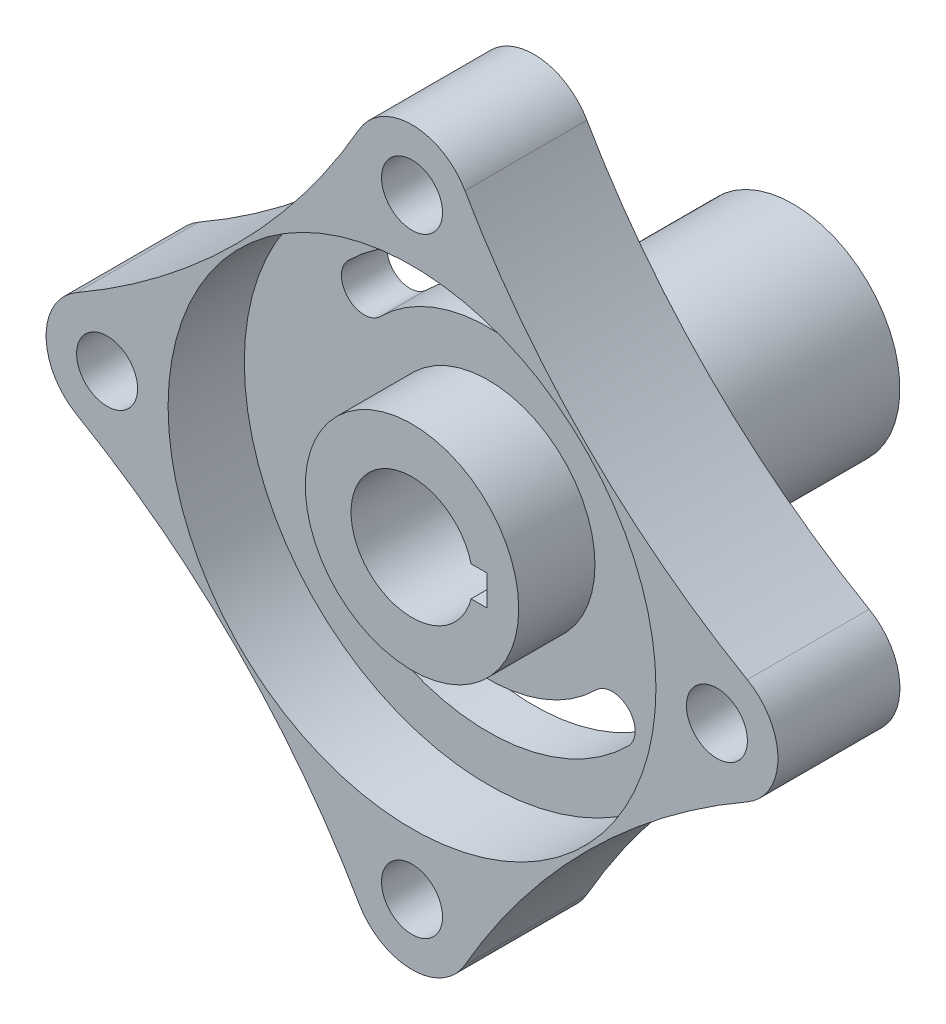
ISO-10303-21;
HEADER;
FILE_DESCRIPTION(('STEP AP214'),'2;1');
FILE_NAME('part.step','',(''),(''),'','','');
FILE_SCHEMA(('AUTOMOTIVE_DESIGN { 1 0 10303 214 1 1 1 1 }'));
ENDSEC;
DATA;
#1=APPLICATION_CONTEXT('core data for automotive mechanical design processes');
#2=APPLICATION_PROTOCOL_DEFINITION('international standard','automotive_design',2000,#1);
#3=PRODUCT_CONTEXT('',#1,'mechanical');
#4=PRODUCT('Part','Part','',(#3));
#5=PRODUCT_RELATED_PRODUCT_CATEGORY('part','',(#4));
#6=PRODUCT_DEFINITION_FORMATION('','',#4);
#7=PRODUCT_DEFINITION_CONTEXT('part definition',#1,'design');
#8=PRODUCT_DEFINITION('design','',#6,#7);
#9=PRODUCT_DEFINITION_SHAPE('','',#8);
#10=(LENGTH_UNIT() NAMED_UNIT(*) SI_UNIT(.MILLI.,.METRE.));
#11=(NAMED_UNIT(*) PLANE_ANGLE_UNIT() SI_UNIT($,.RADIAN.));
#12=(NAMED_UNIT(*) SI_UNIT($,.STERADIAN.) SOLID_ANGLE_UNIT());
#13=UNCERTAINTY_MEASURE_WITH_UNIT(LENGTH_MEASURE(1.E-05),#10,'distance_accuracy_value','');
#14=(GEOMETRIC_REPRESENTATION_CONTEXT(3) GLOBAL_UNCERTAINTY_ASSIGNED_CONTEXT((#13)) GLOBAL_UNIT_ASSIGNED_CONTEXT((#10,
#11,#12)) REPRESENTATION_CONTEXT('',''));
#15=CARTESIAN_POINT('',(0.,0.,0.));
#16=DIRECTION('',(0.,0.,1.));
#17=DIRECTION('',(1.,0.,0.));
#18=AXIS2_PLACEMENT_3D('',#15,#16,#17);
#19=CARTESIAN_POINT('',(0.,0.,0.));
#20=DIRECTION('',(0.,0.,1.));
#21=DIRECTION('',(1.,0.,0.));
#22=AXIS2_PLACEMENT_3D('',#19,#20,#21);
#23=PLANE('',#22);
#24=CARTESIAN_POINT('',(0.,0.,0.));
#25=DIRECTION('',(0.,0.,-1.));
#26=DIRECTION('',(-1.,0.,0.));
#27=AXIS2_PLACEMENT_3D('',#24,#25,#26);
#28=CIRCLE('',#27,14.);
#29=CARTESIAN_POINT('',(-14.,0.,0.));
#30=VERTEX_POINT('',#29);
#31=EDGE_CURVE('E11',#30,#30,#28,.T.);
#32=ORIENTED_EDGE('',*,*,#31,.F.);
#33=EDGE_LOOP('',(#32));
#34=FACE_BOUND('',#33,.T.);
#35=CARTESIAN_POINT('',(-93.7021030907532,-93.7021030907531,0.));
#36=DIRECTION('',(0.,0.,1.));
#37=DIRECTION('',(1.,0.,0.));
#38=AXIS2_PLACEMENT_3D('',#35,#36,#37);
#39=CIRCLE('',#38,100.);
#40=CARTESIAN_POINT('',(-6.94089652524097,-43.977933562278,0.));
#41=VERTEX_POINT('',#40);
#42=CARTESIAN_POINT('',(-43.9779335622782,-6.94089652524068,0.));
#43=VERTEX_POINT('',#42);
#44=EDGE_CURVE('E300',#41,#43,#39,.T.);
#45=ORIENTED_EDGE('',*,*,#44,.T.);
#46=CARTESIAN_POINT('',(-40.,0.,0.));
#47=DIRECTION('',(0.,0.,1.));
#48=DIRECTION('',(1.,0.,0.));
#49=AXIS2_PLACEMENT_3D('',#46,#47,#48);
#50=CIRCLE('',#49,7.99999999999983);
#51=CARTESIAN_POINT('',(-43.9779335622779,6.94089652524083,0.));
#52=VERTEX_POINT('',#51);
#53=EDGE_CURVE('E352',#52,#43,#50,.T.);
#54=ORIENTED_EDGE('',*,*,#53,.F.);
#55=CARTESIAN_POINT('',(-93.7021030907531,93.7021030907531,0.));
#56=DIRECTION('',(0.,0.,1.));
#57=DIRECTION('',(1.,0.,0.));
#58=AXIS2_PLACEMENT_3D('',#55,#56,#57);
#59=CIRCLE('',#58,100.);
#60=CARTESIAN_POINT('',(-6.94089652524097,43.977933562278,0.));
#61=VERTEX_POINT('',#60);
#62=EDGE_CURVE('E353',#52,#61,#59,.T.);
#63=ORIENTED_EDGE('',*,*,#62,.T.);
#64=CARTESIAN_POINT('',(0.,40.,0.));
#65=DIRECTION('',(0.,0.,1.));
#66=DIRECTION('',(1.,0.,0.));
#67=AXIS2_PLACEMENT_3D('',#64,#65,#66);
#68=CIRCLE('',#67,8.);
#69=CARTESIAN_POINT('',(6.94089652524097,43.977933562278,0.));
#70=VERTEX_POINT('',#69);
#71=EDGE_CURVE('E346',#70,#61,#68,.T.);
#72=ORIENTED_EDGE('',*,*,#71,.F.);
#73=CARTESIAN_POINT('',(93.7021030907531,93.7021030907531,0.));
#74=DIRECTION('',(0.,0.,1.));
#75=DIRECTION('',(1.,0.,0.));
#76=AXIS2_PLACEMENT_3D('',#73,#74,#75);
#77=CIRCLE('',#76,100.);
#78=CARTESIAN_POINT('',(43.977933562278,6.94089652524094,0.));
#79=VERTEX_POINT('',#78);
#80=EDGE_CURVE('E344',#70,#79,#77,.T.);
#81=ORIENTED_EDGE('',*,*,#80,.T.);
#82=CARTESIAN_POINT('',(40.,0.,0.));
#83=DIRECTION('',(0.,0.,1.));
#84=DIRECTION('',(1.,0.,0.));
#85=AXIS2_PLACEMENT_3D('',#82,#83,#84);
#86=CIRCLE('',#85,7.99999999999997);
#87=CARTESIAN_POINT('',(43.977933562278,-6.94089652524095,0.));
#88=VERTEX_POINT('',#87);
#89=EDGE_CURVE('E345',#88,#79,#86,.T.);
#90=ORIENTED_EDGE('',*,*,#89,.F.);
#91=CARTESIAN_POINT('',(93.7021030907531,-93.7021030907531,0.));
#92=DIRECTION('',(0.,0.,1.));
#93=DIRECTION('',(1.,0.,0.));
#94=AXIS2_PLACEMENT_3D('',#91,#92,#93);
#95=CIRCLE('',#94,100.);
#96=CARTESIAN_POINT('',(6.94089652524096,-43.977933562278,0.));
#97=VERTEX_POINT('',#96);
#98=EDGE_CURVE('E337',#88,#97,#95,.T.);
#99=ORIENTED_EDGE('',*,*,#98,.T.);
#100=CARTESIAN_POINT('',(0.,-40.,0.));
#101=DIRECTION('',(0.,0.,1.));
#102=DIRECTION('',(1.,0.,0.));
#103=AXIS2_PLACEMENT_3D('',#100,#101,#102);
#104=CIRCLE('',#103,8.);
#105=EDGE_CURVE('E338',#41,#97,#104,.T.);
#106=ORIENTED_EDGE('',*,*,#105,.F.);
#107=EDGE_LOOP('',(#45,#54,#63,#72,#81,#90,#99,#106));
#108=FACE_BOUND('',#107,.T.);
#109=CARTESIAN_POINT('',(0.,-40.,0.));
#110=DIRECTION('',(0.,0.,1.));
#111=DIRECTION('',(1.,0.,0.));
#112=AXIS2_PLACEMENT_3D('',#109,#110,#111);
#113=CIRCLE('',#112,4.);
#114=CARTESIAN_POINT('',(4.,-40.,0.));
#115=VERTEX_POINT('',#114);
#116=EDGE_CURVE('E360',#115,#115,#113,.T.);
#117=ORIENTED_EDGE('',*,*,#116,.T.);
#118=EDGE_LOOP('',(#117));
#119=FACE_BOUND('',#118,.T.);
#120=CARTESIAN_POINT('',(-40.,0.,0.));
#121=DIRECTION('',(0.,0.,1.));
#122=DIRECTION('',(1.,0.,0.));
#123=AXIS2_PLACEMENT_3D('',#120,#121,#122);
#124=CIRCLE('',#123,4.);
#125=CARTESIAN_POINT('',(-36.,0.,0.));
#126=VERTEX_POINT('',#125);
#127=EDGE_CURVE('E359',#126,#126,#124,.T.);
#128=ORIENTED_EDGE('',*,*,#127,.T.);
#129=EDGE_LOOP('',(#128));
#130=FACE_BOUND('',#129,.T.);
#131=CARTESIAN_POINT('',(40.,0.,0.));
#132=DIRECTION('',(0.,0.,1.));
#133=DIRECTION('',(1.,0.,0.));
#134=AXIS2_PLACEMENT_3D('',#131,#132,#133);
#135=CIRCLE('',#134,4.);
#136=CARTESIAN_POINT('',(44.,0.,0.));
#137=VERTEX_POINT('',#136);
#138=EDGE_CURVE('E361',#137,#137,#135,.T.);
#139=ORIENTED_EDGE('',*,*,#138,.T.);
#140=EDGE_LOOP('',(#139));
#141=FACE_BOUND('',#140,.T.);
#142=CARTESIAN_POINT('',(0.,40.,0.));
#143=DIRECTION('',(0.,0.,1.));
#144=DIRECTION('',(1.,0.,0.));
#145=AXIS2_PLACEMENT_3D('',#142,#143,#144);
#146=CIRCLE('',#145,4.);
#147=CARTESIAN_POINT('',(4.,40.,0.));
#148=VERTEX_POINT('',#147);
#149=EDGE_CURVE('E302',#148,#148,#146,.T.);
#150=ORIENTED_EDGE('',*,*,#149,.T.);
#151=EDGE_LOOP('',(#150));
#152=FACE_BOUND('',#151,.T.);
#153=CARTESIAN_POINT('',(0.,0.,0.));
#154=DIRECTION('',(0.,0.,1.));
#155=DIRECTION('',(1.,0.,0.));
#156=AXIS2_PLACEMENT_3D('',#153,#154,#155);
#157=CIRCLE('',#156,26.);
#158=CARTESIAN_POINT('',(18.3847763108502,18.3847763108503,0.));
#159=VERTEX_POINT('',#158);
#160=CARTESIAN_POINT('',(-18.3847763108502,18.3847763108503,0.));
#161=VERTEX_POINT('',#160);
#162=EDGE_CURVE('E273',#159,#161,#157,.T.);
#163=ORIENTED_EDGE('',*,*,#162,.T.);
#164=CARTESIAN_POINT('',(-16.2634559672906,16.2634559672906,0.));
#165=DIRECTION('',(0.,0.,1.));
#166=DIRECTION('',(1.,0.,0.));
#167=AXIS2_PLACEMENT_3D('',#164,#165,#166);
#168=CIRCLE('',#167,3.);
#169=CARTESIAN_POINT('',(-14.1421356237309,14.142135623731,0.));
#170=VERTEX_POINT('',#169);
#171=EDGE_CURVE('E262',#161,#170,#168,.T.);
#172=ORIENTED_EDGE('',*,*,#171,.T.);
#173=CARTESIAN_POINT('',(0.,0.,0.));
#174=DIRECTION('',(0.,0.,-1.));
#175=DIRECTION('',(1.,0.,0.));
#176=AXIS2_PLACEMENT_3D('',#173,#174,#175);
#177=CIRCLE('',#176,20.);
#178=CARTESIAN_POINT('',(14.1421356237309,14.142135623731,0.));
#179=VERTEX_POINT('',#178);
#180=EDGE_CURVE('E270',#170,#179,#177,.T.);
#181=ORIENTED_EDGE('',*,*,#180,.T.);
#182=CARTESIAN_POINT('',(16.2634559672906,16.2634559672906,0.));
#183=DIRECTION('',(0.,0.,1.));
#184=DIRECTION('',(1.,0.,0.));
#185=AXIS2_PLACEMENT_3D('',#182,#183,#184);
#186=CIRCLE('',#185,3.);
#187=EDGE_CURVE('E271',#179,#159,#186,.T.);
#188=ORIENTED_EDGE('',*,*,#187,.T.);
#189=EDGE_LOOP('',(#163,#172,#181,#188));
#190=FACE_BOUND('',#189,.T.);
#191=CARTESIAN_POINT('',(0.,0.,0.));
#192=DIRECTION('',(0.,0.,-1.));
#193=DIRECTION('',(1.,0.,0.));
#194=AXIS2_PLACEMENT_3D('',#191,#192,#193);
#195=CIRCLE('',#194,20.);
#196=CARTESIAN_POINT('',(14.1421356237309,-14.142135623731,0.));
#197=VERTEX_POINT('',#196);
#198=CARTESIAN_POINT('',(-14.1421356237309,-14.142135623731,0.));
#199=VERTEX_POINT('',#198);
#200=EDGE_CURVE('E238',#197,#199,#195,.T.);
#201=ORIENTED_EDGE('',*,*,#200,.T.);
#202=CARTESIAN_POINT('',(-16.2634559672906,-16.2634559672906,0.));
#203=DIRECTION('',(0.,0.,1.));
#204=DIRECTION('',(-1.,0.,0.));
#205=AXIS2_PLACEMENT_3D('',#202,#203,#204);
#206=CIRCLE('',#205,3.);
#207=CARTESIAN_POINT('',(-18.3847763108502,-18.3847763108503,0.));
#208=VERTEX_POINT('',#207);
#209=EDGE_CURVE('E235',#199,#208,#206,.T.);
#210=ORIENTED_EDGE('',*,*,#209,.T.);
#211=CARTESIAN_POINT('',(0.,0.,0.));
#212=DIRECTION('',(0.,0.,1.));
#213=DIRECTION('',(1.,0.,0.));
#214=AXIS2_PLACEMENT_3D('',#211,#212,#213);
#215=CIRCLE('',#214,26.);
#216=CARTESIAN_POINT('',(18.3847763108502,-18.3847763108503,0.));
#217=VERTEX_POINT('',#216);
#218=EDGE_CURVE('E234',#208,#217,#215,.T.);
#219=ORIENTED_EDGE('',*,*,#218,.T.);
#220=CARTESIAN_POINT('',(16.2634559672906,-16.2634559672906,0.));
#221=DIRECTION('',(0.,0.,1.));
#222=DIRECTION('',(1.,0.,0.));
#223=AXIS2_PLACEMENT_3D('',#220,#221,#222);
#224=CIRCLE('',#223,3.);
#225=EDGE_CURVE('E72',#217,#197,#224,.T.);
#226=ORIENTED_EDGE('',*,*,#225,.T.);
#227=EDGE_LOOP('',(#201,#210,#219,#226));
#228=FACE_BOUND('',#227,.T.);
#229=ADVANCED_FACE('F50',(#34,#108,#119,#130,#141,#152,#190,#228),#23,.F.);
#230=CARTESIAN_POINT('',(0.,0.,6.));
#231=DIRECTION('',(0.,0.,1.));
#232=DIRECTION('',(1.,0.,0.));
#233=AXIS2_PLACEMENT_3D('',#230,#231,#232);
#234=PLANE('',#233);
#235=CARTESIAN_POINT('',(0.,0.,6.));
#236=DIRECTION('',(0.,0.,1.));
#237=DIRECTION('',(1.,0.,0.));
#238=AXIS2_PLACEMENT_3D('',#235,#236,#237);
#239=CIRCLE('',#238,14.);
#240=CARTESIAN_POINT('',(14.,0.,6.));
#241=VERTEX_POINT('',#240);
#242=EDGE_CURVE('E221',#241,#241,#239,.T.);
#243=ORIENTED_EDGE('',*,*,#242,.F.);
#244=EDGE_LOOP('',(#243));
#245=FACE_BOUND('',#244,.T.);
#246=CARTESIAN_POINT('',(-16.2634559672906,16.2634559672906,6.));
#247=DIRECTION('',(0.,0.,1.));
#248=DIRECTION('',(1.,0.,0.));
#249=AXIS2_PLACEMENT_3D('',#246,#247,#248);
#250=CIRCLE('',#249,3.);
#251=CARTESIAN_POINT('',(-18.3847763108502,18.3847763108503,6.));
#252=VERTEX_POINT('',#251);
#253=CARTESIAN_POINT('',(-14.1421356237309,14.142135623731,6.));
#254=VERTEX_POINT('',#253);
#255=EDGE_CURVE('E227',#252,#254,#250,.T.);
#256=ORIENTED_EDGE('',*,*,#255,.F.);
#257=CARTESIAN_POINT('',(0.,0.,6.));
#258=DIRECTION('',(0.,0.,1.));
#259=DIRECTION('',(1.,0.,0.));
#260=AXIS2_PLACEMENT_3D('',#257,#258,#259);
#261=CIRCLE('',#260,26.);
#262=CARTESIAN_POINT('',(18.3847763108502,18.3847763108503,6.));
#263=VERTEX_POINT('',#262);
#264=EDGE_CURVE('E268',#263,#252,#261,.T.);
#265=ORIENTED_EDGE('',*,*,#264,.F.);
#266=CARTESIAN_POINT('',(16.2634559672906,16.2634559672906,6.));
#267=DIRECTION('',(0.,0.,1.));
#268=DIRECTION('',(1.,0.,0.));
#269=AXIS2_PLACEMENT_3D('',#266,#267,#268);
#270=CIRCLE('',#269,3.);
#271=CARTESIAN_POINT('',(14.1421356237309,14.142135623731,6.));
#272=VERTEX_POINT('',#271);
#273=EDGE_CURVE('E285',#272,#263,#270,.T.);
#274=ORIENTED_EDGE('',*,*,#273,.F.);
#275=CARTESIAN_POINT('',(0.,0.,6.));
#276=DIRECTION('',(0.,0.,-1.));
#277=DIRECTION('',(1.,0.,0.));
#278=AXIS2_PLACEMENT_3D('',#275,#276,#277);
#279=CIRCLE('',#278,20.);
#280=EDGE_CURVE('E276',#254,#272,#279,.T.);
#281=ORIENTED_EDGE('',*,*,#280,.F.);
#282=EDGE_LOOP('',(#256,#265,#274,#281));
#283=FACE_BOUND('',#282,.T.);
#284=CARTESIAN_POINT('',(0.,0.,6.));
#285=DIRECTION('',(0.,0.,1.));
#286=DIRECTION('',(1.,0.,0.));
#287=AXIS2_PLACEMENT_3D('',#284,#285,#286);
#288=CIRCLE('',#287,32.);
#289=CARTESIAN_POINT('',(32.,0.,6.));
#290=VERTEX_POINT('',#289);
#291=EDGE_CURVE('E294',#290,#290,#288,.T.);
#292=ORIENTED_EDGE('',*,*,#291,.T.);
#293=EDGE_LOOP('',(#292));
#294=FACE_BOUND('',#293,.T.);
#295=CARTESIAN_POINT('',(-16.2634559672906,-16.2634559672906,6.));
#296=DIRECTION('',(0.,0.,1.));
#297=DIRECTION('',(-1.,0.,0.));
#298=AXIS2_PLACEMENT_3D('',#295,#296,#297);
#299=CIRCLE('',#298,3.);
#300=CARTESIAN_POINT('',(-14.1421356237309,-14.142135623731,6.));
#301=VERTEX_POINT('',#300);
#302=CARTESIAN_POINT('',(-18.3847763108502,-18.3847763108503,6.));
#303=VERTEX_POINT('',#302);
#304=EDGE_CURVE('E242',#301,#303,#299,.T.);
#305=ORIENTED_EDGE('',*,*,#304,.F.);
#306=CARTESIAN_POINT('',(0.,0.,6.));
#307=DIRECTION('',(0.,0.,-1.));
#308=DIRECTION('',(1.,0.,0.));
#309=AXIS2_PLACEMENT_3D('',#306,#307,#308);
#310=CIRCLE('',#309,20.);
#311=CARTESIAN_POINT('',(14.1421356237309,-14.142135623731,6.));
#312=VERTEX_POINT('',#311);
#313=EDGE_CURVE('E237',#312,#301,#310,.T.);
#314=ORIENTED_EDGE('',*,*,#313,.F.);
#315=CARTESIAN_POINT('',(16.2634559672906,-16.2634559672906,6.));
#316=DIRECTION('',(0.,0.,1.));
#317=DIRECTION('',(1.,0.,0.));
#318=AXIS2_PLACEMENT_3D('',#315,#316,#317);
#319=CIRCLE('',#318,3.);
#320=CARTESIAN_POINT('',(18.3847763108502,-18.3847763108503,6.));
#321=VERTEX_POINT('',#320);
#322=EDGE_CURVE('E249',#321,#312,#319,.T.);
#323=ORIENTED_EDGE('',*,*,#322,.F.);
#324=CARTESIAN_POINT('',(0.,0.,6.));
#325=DIRECTION('',(0.,0.,1.));
#326=DIRECTION('',(1.,0.,0.));
#327=AXIS2_PLACEMENT_3D('',#324,#325,#326);
#328=CIRCLE('',#327,26.);
#329=EDGE_CURVE('E246',#303,#321,#328,.T.);
#330=ORIENTED_EDGE('',*,*,#329,.F.);
#331=EDGE_LOOP('',(#305,#314,#323,#330));
#332=FACE_BOUND('',#331,.T.);
#333=ADVANCED_FACE('F438',(#245,#283,#294,#332),#234,.T.);
#334=CARTESIAN_POINT('',(-93.7021030907532,-93.7021030907531,16.));
#335=DIRECTION('',(0.,0.,-1.));
#336=DIRECTION('',(-1.,0.,0.));
#337=AXIS2_PLACEMENT_3D('',#334,#335,#336);
#338=CYLINDRICAL_SURFACE('',#337,100.);
#339=ORIENTED_EDGE('',*,*,#44,.F.);
#340=DIRECTION('',(0.,0.,-1.));
#341=VECTOR('',#340,1.);
#342=CARTESIAN_POINT('',(-6.94089652524097,-43.977933562278,16.));
#343=LINE('',#342,#341);
#344=CARTESIAN_POINT('',(-6.94089652524097,-43.977933562278,16.));
#345=VERTEX_POINT('',#344);
#346=EDGE_CURVE('E51',#345,#41,#343,.T.);
#347=ORIENTED_EDGE('',*,*,#346,.F.);
#348=CARTESIAN_POINT('',(-93.7021030907532,-93.7021030907531,16.));
#349=DIRECTION('',(0.,0.,1.));
#350=DIRECTION('',(1.,0.,0.));
#351=AXIS2_PLACEMENT_3D('',#348,#349,#350);
#352=CIRCLE('',#351,100.);
#353=CARTESIAN_POINT('',(-43.9779335622782,-6.94089652524068,16.));
#354=VERTEX_POINT('',#353);
#355=EDGE_CURVE('E299',#345,#354,#352,.T.);
#356=ORIENTED_EDGE('',*,*,#355,.T.);
#357=DIRECTION('',(0.,0.,-1.));
#358=VECTOR('',#357,1.);
#359=CARTESIAN_POINT('',(-43.9779335622782,-6.94089652524068,16.));
#360=LINE('',#359,#358);
#361=EDGE_CURVE('E334',#354,#43,#360,.T.);
#362=ORIENTED_EDGE('',*,*,#361,.T.);
#363=EDGE_LOOP('',(#339,#347,#356,#362));
#364=FACE_BOUND('',#363,.T.);
#365=ADVANCED_FACE('F47',(#364),#338,.F.);
#366=CARTESIAN_POINT('',(0.,-40.,16.));
#367=DIRECTION('',(0.,0.,-1.));
#368=DIRECTION('',(-1.,0.,0.));
#369=AXIS2_PLACEMENT_3D('',#366,#367,#368);
#370=CYLINDRICAL_SURFACE('',#369,8.);
#371=ORIENTED_EDGE('',*,*,#105,.T.);
#372=DIRECTION('',(0.,0.,-1.));
#373=VECTOR('',#372,1.);
#374=CARTESIAN_POINT('',(6.94089652524096,-43.977933562278,16.));
#375=LINE('',#374,#373);
#376=CARTESIAN_POINT('',(6.94089652524096,-43.977933562278,16.));
#377=VERTEX_POINT('',#376);
#378=EDGE_CURVE('E378',#377,#97,#375,.T.);
#379=ORIENTED_EDGE('',*,*,#378,.F.);
#380=CARTESIAN_POINT('',(0.,-40.,16.));
#381=DIRECTION('',(0.,0.,1.));
#382=DIRECTION('',(1.,0.,0.));
#383=AXIS2_PLACEMENT_3D('',#380,#381,#382);
#384=CIRCLE('',#383,8.);
#385=EDGE_CURVE('E303',#345,#377,#384,.T.);
#386=ORIENTED_EDGE('',*,*,#385,.F.);
#387=ORIENTED_EDGE('',*,*,#346,.T.);
#388=EDGE_LOOP('',(#371,#379,#386,#387));
#389=FACE_BOUND('',#388,.T.);
#390=ADVANCED_FACE('F384',(#389),#370,.T.);
#391=CARTESIAN_POINT('',(93.7021030907531,-93.7021030907531,16.));
#392=DIRECTION('',(0.,0.,-1.));
#393=DIRECTION('',(-1.,0.,0.));
#394=AXIS2_PLACEMENT_3D('',#391,#392,#393);
#395=CYLINDRICAL_SURFACE('',#394,100.);
#396=ORIENTED_EDGE('',*,*,#98,.F.);
#397=DIRECTION('',(0.,0.,-1.));
#398=VECTOR('',#397,1.);
#399=CARTESIAN_POINT('',(43.977933562278,-6.94089652524095,16.));
#400=LINE('',#399,#398);
#401=CARTESIAN_POINT('',(43.977933562278,-6.94089652524095,16.));
#402=VERTEX_POINT('',#401);
#403=EDGE_CURVE('E380',#402,#88,#400,.T.);
#404=ORIENTED_EDGE('',*,*,#403,.F.);
#405=CARTESIAN_POINT('',(93.7021030907531,-93.7021030907531,16.));
#406=DIRECTION('',(0.,0.,1.));
#407=DIRECTION('',(1.,0.,0.));
#408=AXIS2_PLACEMENT_3D('',#405,#406,#407);
#409=CIRCLE('',#408,100.);
#410=EDGE_CURVE('E308',#402,#377,#409,.T.);
#411=ORIENTED_EDGE('',*,*,#410,.T.);
#412=ORIENTED_EDGE('',*,*,#378,.T.);
#413=EDGE_LOOP('',(#396,#404,#411,#412));
#414=FACE_BOUND('',#413,.T.);
#415=ADVANCED_FACE('F412',(#414),#395,.F.);
#416=CARTESIAN_POINT('',(40.,0.,16.));
#417=DIRECTION('',(0.,0.,-1.));
#418=DIRECTION('',(-1.,0.,0.));
#419=AXIS2_PLACEMENT_3D('',#416,#417,#418);
#420=CYLINDRICAL_SURFACE('',#419,7.99999999999997);
#421=ORIENTED_EDGE('',*,*,#89,.T.);
#422=DIRECTION('',(0.,0.,-1.));
#423=VECTOR('',#422,1.);
#424=CARTESIAN_POINT('',(43.977933562278,6.94089652524094,16.));
#425=LINE('',#424,#423);
#426=CARTESIAN_POINT('',(43.977933562278,6.94089652524094,16.));
#427=VERTEX_POINT('',#426);
#428=EDGE_CURVE('E374',#427,#79,#425,.T.);
#429=ORIENTED_EDGE('',*,*,#428,.F.);
#430=CARTESIAN_POINT('',(40.,0.,16.));
#431=DIRECTION('',(0.,0.,1.));
#432=DIRECTION('',(1.,0.,0.));
#433=AXIS2_PLACEMENT_3D('',#430,#431,#432);
#434=CIRCLE('',#433,7.99999999999997);
#435=EDGE_CURVE('E310',#402,#427,#434,.T.);
#436=ORIENTED_EDGE('',*,*,#435,.F.);
#437=ORIENTED_EDGE('',*,*,#403,.T.);
#438=EDGE_LOOP('',(#421,#429,#436,#437));
#439=FACE_BOUND('',#438,.T.);
#440=ADVANCED_FACE('F413',(#439),#420,.T.);
#441=CARTESIAN_POINT('',(93.7021030907531,93.7021030907531,16.));
#442=DIRECTION('',(0.,0.,-1.));
#443=DIRECTION('',(-1.,0.,0.));
#444=AXIS2_PLACEMENT_3D('',#441,#442,#443);
#445=CYLINDRICAL_SURFACE('',#444,100.);
#446=ORIENTED_EDGE('',*,*,#80,.F.);
#447=DIRECTION('',(0.,0.,-1.));
#448=VECTOR('',#447,1.);
#449=CARTESIAN_POINT('',(6.94089652524097,43.977933562278,16.));
#450=LINE('',#449,#448);
#451=CARTESIAN_POINT('',(6.94089652524097,43.977933562278,16.));
#452=VERTEX_POINT('',#451);
#453=EDGE_CURVE('E373',#452,#70,#450,.T.);
#454=ORIENTED_EDGE('',*,*,#453,.F.);
#455=CARTESIAN_POINT('',(93.7021030907531,93.7021030907531,16.));
#456=DIRECTION('',(0.,0.,1.));
#457=DIRECTION('',(1.,0.,0.));
#458=AXIS2_PLACEMENT_3D('',#455,#456,#457);
#459=CIRCLE('',#458,100.);
#460=EDGE_CURVE('E313',#452,#427,#459,.T.);
#461=ORIENTED_EDGE('',*,*,#460,.T.);
#462=ORIENTED_EDGE('',*,*,#428,.T.);
#463=EDGE_LOOP('',(#446,#454,#461,#462));
#464=FACE_BOUND('',#463,.T.);
#465=ADVANCED_FACE('F406',(#464),#445,.F.);
#466=CARTESIAN_POINT('',(0.,40.,16.));
#467=DIRECTION('',(0.,0.,-1.));
#468=DIRECTION('',(-1.,0.,0.));
#469=AXIS2_PLACEMENT_3D('',#466,#467,#468);
#470=CYLINDRICAL_SURFACE('',#469,8.);
#471=ORIENTED_EDGE('',*,*,#71,.T.);
#472=DIRECTION('',(0.,0.,-1.));
#473=VECTOR('',#472,1.);
#474=CARTESIAN_POINT('',(-6.94089652524097,43.977933562278,16.));
#475=LINE('',#474,#473);
#476=CARTESIAN_POINT('',(-6.94089652524097,43.977933562278,16.));
#477=VERTEX_POINT('',#476);
#478=EDGE_CURVE('E371',#477,#61,#475,.T.);
#479=ORIENTED_EDGE('',*,*,#478,.F.);
#480=CARTESIAN_POINT('',(0.,40.,16.));
#481=DIRECTION('',(0.,0.,1.));
#482=DIRECTION('',(1.,0.,0.));
#483=AXIS2_PLACEMENT_3D('',#480,#481,#482);
#484=CIRCLE('',#483,8.);
#485=EDGE_CURVE('E314',#452,#477,#484,.T.);
#486=ORIENTED_EDGE('',*,*,#485,.F.);
#487=ORIENTED_EDGE('',*,*,#453,.T.);
#488=EDGE_LOOP('',(#471,#479,#486,#487));
#489=FACE_BOUND('',#488,.T.);
#490=ADVANCED_FACE('F403',(#489),#470,.T.);
#491=CARTESIAN_POINT('',(-93.7021030907531,93.7021030907531,16.));
#492=DIRECTION('',(0.,0.,-1.));
#493=DIRECTION('',(-1.,0.,0.));
#494=AXIS2_PLACEMENT_3D('',#491,#492,#493);
#495=CYLINDRICAL_SURFACE('',#494,100.);
#496=ORIENTED_EDGE('',*,*,#62,.F.);
#497=DIRECTION('',(0.,0.,-1.));
#498=VECTOR('',#497,1.);
#499=CARTESIAN_POINT('',(-43.9779335622779,6.94089652524083,16.));
#500=LINE('',#499,#498);
#501=CARTESIAN_POINT('',(-43.9779335622779,6.94089652524083,16.));
#502=VERTEX_POINT('',#501);
#503=EDGE_CURVE('E369',#502,#52,#500,.T.);
#504=ORIENTED_EDGE('',*,*,#503,.F.);
#505=CARTESIAN_POINT('',(-93.7021030907531,93.7021030907531,16.));
#506=DIRECTION('',(0.,0.,1.));
#507=DIRECTION('',(1.,0.,0.));
#508=AXIS2_PLACEMENT_3D('',#505,#506,#507);
#509=CIRCLE('',#508,100.);
#510=EDGE_CURVE('E316',#502,#477,#509,.T.);
#511=ORIENTED_EDGE('',*,*,#510,.T.);
#512=ORIENTED_EDGE('',*,*,#478,.T.);
#513=EDGE_LOOP('',(#496,#504,#511,#512));
#514=FACE_BOUND('',#513,.T.);
#515=ADVANCED_FACE('F399',(#514),#495,.F.);
#516=CARTESIAN_POINT('',(40.,0.,16.));
#517=DIRECTION('',(0.,0.,-1.));
#518=DIRECTION('',(-1.,0.,0.));
#519=AXIS2_PLACEMENT_3D('',#516,#517,#518);
#520=CYLINDRICAL_SURFACE('',#519,4.);
#521=CARTESIAN_POINT('',(40.,0.,16.));
#522=DIRECTION('',(0.,0.,1.));
#523=DIRECTION('',(1.,0.,0.));
#524=AXIS2_PLACEMENT_3D('',#521,#522,#523);
#525=CIRCLE('',#524,4.);
#526=CARTESIAN_POINT('',(44.,0.,16.));
#527=VERTEX_POINT('',#526);
#528=EDGE_CURVE('E330',#527,#527,#525,.T.);
#529=ORIENTED_EDGE('',*,*,#528,.T.);
#530=EDGE_LOOP('',(#529));
#531=FACE_BOUND('',#530,.T.);
#532=ORIENTED_EDGE('',*,*,#138,.F.);
#533=EDGE_LOOP('',(#532));
#534=FACE_BOUND('',#533,.T.);
#535=ADVANCED_FACE('F478',(#531,#534),#520,.F.);
#536=CARTESIAN_POINT('',(-40.,0.,16.));
#537=DIRECTION('',(0.,0.,-1.));
#538=DIRECTION('',(-1.,0.,0.));
#539=AXIS2_PLACEMENT_3D('',#536,#537,#538);
#540=CYLINDRICAL_SURFACE('',#539,4.);
#541=CARTESIAN_POINT('',(-40.,0.,16.));
#542=DIRECTION('',(0.,0.,1.));
#543=DIRECTION('',(1.,0.,0.));
#544=AXIS2_PLACEMENT_3D('',#541,#542,#543);
#545=CIRCLE('',#544,4.);
#546=CARTESIAN_POINT('',(-36.,0.,16.));
#547=VERTEX_POINT('',#546);
#548=EDGE_CURVE('E322',#547,#547,#545,.T.);
#549=ORIENTED_EDGE('',*,*,#548,.T.);
#550=EDGE_LOOP('',(#549));
#551=FACE_BOUND('',#550,.T.);
#552=ORIENTED_EDGE('',*,*,#127,.F.);
#553=EDGE_LOOP('',(#552));
#554=FACE_BOUND('',#553,.T.);
#555=ADVANCED_FACE('F479',(#551,#554),#540,.F.);
#556=CARTESIAN_POINT('',(0.,-40.,16.));
#557=DIRECTION('',(0.,0.,-1.));
#558=DIRECTION('',(-1.,0.,0.));
#559=AXIS2_PLACEMENT_3D('',#556,#557,#558);
#560=CYLINDRICAL_SURFACE('',#559,4.);
#561=CARTESIAN_POINT('',(0.,-40.,16.));
#562=DIRECTION('',(0.,0.,1.));
#563=DIRECTION('',(1.,0.,0.));
#564=AXIS2_PLACEMENT_3D('',#561,#562,#563);
#565=CIRCLE('',#564,4.);
#566=CARTESIAN_POINT('',(4.,-40.,16.));
#567=VERTEX_POINT('',#566);
#568=EDGE_CURVE('E321',#567,#567,#565,.T.);
#569=ORIENTED_EDGE('',*,*,#568,.T.);
#570=EDGE_LOOP('',(#569));
#571=FACE_BOUND('',#570,.T.);
#572=ORIENTED_EDGE('',*,*,#116,.F.);
#573=EDGE_LOOP('',(#572));
#574=FACE_BOUND('',#573,.T.);
#575=ADVANCED_FACE('F483',(#571,#574),#560,.F.);
#576=CARTESIAN_POINT('',(-40.,0.,16.));
#577=DIRECTION('',(0.,0.,-1.));
#578=DIRECTION('',(-1.,0.,0.));
#579=AXIS2_PLACEMENT_3D('',#576,#577,#578);
#580=CYLINDRICAL_SURFACE('',#579,7.99999999999983);
#581=ORIENTED_EDGE('',*,*,#53,.T.);
#582=ORIENTED_EDGE('',*,*,#361,.F.);
#583=CARTESIAN_POINT('',(-40.,0.,16.));
#584=DIRECTION('',(0.,0.,1.));
#585=DIRECTION('',(1.,0.,0.));
#586=AXIS2_PLACEMENT_3D('',#583,#584,#585);
#587=CIRCLE('',#586,7.99999999999983);
#588=EDGE_CURVE('E317',#502,#354,#587,.T.);
#589=ORIENTED_EDGE('',*,*,#588,.F.);
#590=ORIENTED_EDGE('',*,*,#503,.T.);
#591=EDGE_LOOP('',(#581,#582,#589,#590));
#592=FACE_BOUND('',#591,.T.);
#593=ADVANCED_FACE('F396',(#592),#580,.T.);
#594=CARTESIAN_POINT('',(0.,40.,16.));
#595=DIRECTION('',(0.,0.,-1.));
#596=DIRECTION('',(-1.,0.,0.));
#597=AXIS2_PLACEMENT_3D('',#594,#595,#596);
#598=CYLINDRICAL_SURFACE('',#597,4.);
#599=CARTESIAN_POINT('',(0.,40.,16.));
#600=DIRECTION('',(0.,0.,1.));
#601=DIRECTION('',(1.,0.,0.));
#602=AXIS2_PLACEMENT_3D('',#599,#600,#601);
#603=CIRCLE('',#602,4.);
#604=CARTESIAN_POINT('',(4.,40.,16.));
#605=VERTEX_POINT('',#604);
#606=EDGE_CURVE('E329',#605,#605,#603,.T.);
#607=ORIENTED_EDGE('',*,*,#606,.T.);
#608=EDGE_LOOP('',(#607));
#609=FACE_BOUND('',#608,.T.);
#610=ORIENTED_EDGE('',*,*,#149,.F.);
#611=EDGE_LOOP('',(#610));
#612=FACE_BOUND('',#611,.T.);
#613=ADVANCED_FACE('F423',(#609,#612),#598,.F.);
#614=CARTESIAN_POINT('',(0.,0.,16.));
#615=DIRECTION('',(0.,0.,1.));
#616=DIRECTION('',(1.,0.,0.));
#617=AXIS2_PLACEMENT_3D('',#614,#615,#616);
#618=PLANE('',#617);
#619=CARTESIAN_POINT('',(0.,0.,16.));
#620=DIRECTION('',(0.,0.,1.));
#621=DIRECTION('',(1.,0.,0.));
#622=AXIS2_PLACEMENT_3D('',#619,#620,#621);
#623=CIRCLE('',#622,32.);
#624=CARTESIAN_POINT('',(32.,0.,16.));
#625=VERTEX_POINT('',#624);
#626=EDGE_CURVE('E260',#625,#625,#623,.T.);
#627=ORIENTED_EDGE('',*,*,#626,.F.);
#628=EDGE_LOOP('',(#627));
#629=FACE_BOUND('',#628,.T.);
#630=ORIENTED_EDGE('',*,*,#355,.F.);
#631=ORIENTED_EDGE('',*,*,#385,.T.);
#632=ORIENTED_EDGE('',*,*,#410,.F.);
#633=ORIENTED_EDGE('',*,*,#435,.T.);
#634=ORIENTED_EDGE('',*,*,#460,.F.);
#635=ORIENTED_EDGE('',*,*,#485,.T.);
#636=ORIENTED_EDGE('',*,*,#510,.F.);
#637=ORIENTED_EDGE('',*,*,#588,.T.);
#638=EDGE_LOOP('',(#630,#631,#632,#633,#634,#635,#636,#637));
#639=FACE_BOUND('',#638,.T.);
#640=ORIENTED_EDGE('',*,*,#568,.F.);
#641=EDGE_LOOP('',(#640));
#642=FACE_BOUND('',#641,.T.);
#643=ORIENTED_EDGE('',*,*,#548,.F.);
#644=EDGE_LOOP('',(#643));
#645=FACE_BOUND('',#644,.T.);
#646=ORIENTED_EDGE('',*,*,#528,.F.);
#647=EDGE_LOOP('',(#646));
#648=FACE_BOUND('',#647,.T.);
#649=ORIENTED_EDGE('',*,*,#606,.F.);
#650=EDGE_LOOP('',(#649));
#651=FACE_BOUND('',#650,.T.);
#652=ADVANCED_FACE('F417',(#629,#639,#642,#645,#648,#651),#618,.T.);
#653=CARTESIAN_POINT('',(0.,0.,6.));
#654=DIRECTION('',(0.,0.,1.));
#655=DIRECTION('',(1.,0.,0.));
#656=AXIS2_PLACEMENT_3D('',#653,#654,#655);
#657=CYLINDRICAL_SURFACE('',#656,32.);
#658=ORIENTED_EDGE('',*,*,#291,.F.);
#659=EDGE_LOOP('',(#658));
#660=FACE_BOUND('',#659,.T.);
#661=ORIENTED_EDGE('',*,*,#626,.T.);
#662=EDGE_LOOP('',(#661));
#663=FACE_BOUND('',#662,.T.);
#664=ADVANCED_FACE('F419',(#660,#663),#657,.F.);
#665=CARTESIAN_POINT('',(-16.2634559672906,16.2634559672906,0.));
#666=DIRECTION('',(0.,0.,1.));
#667=DIRECTION('',(1.,0.,0.));
#668=AXIS2_PLACEMENT_3D('',#665,#666,#667);
#669=CYLINDRICAL_SURFACE('',#668,3.);
#670=ORIENTED_EDGE('',*,*,#255,.T.);
#671=DIRECTION('',(0.,0.,1.));
#672=VECTOR('',#671,1.);
#673=CARTESIAN_POINT('',(-14.1421356237309,14.142135623731,0.));
#674=LINE('',#673,#672);
#675=EDGE_CURVE('E280',#170,#254,#674,.T.);
#676=ORIENTED_EDGE('',*,*,#675,.F.);
#677=ORIENTED_EDGE('',*,*,#171,.F.);
#678=DIRECTION('',(0.,0.,1.));
#679=VECTOR('',#678,1.);
#680=CARTESIAN_POINT('',(-18.3847763108502,18.3847763108503,0.));
#681=LINE('',#680,#679);
#682=EDGE_CURVE('E250',#161,#252,#681,.T.);
#683=ORIENTED_EDGE('',*,*,#682,.T.);
#684=EDGE_LOOP('',(#670,#676,#677,#683));
#685=FACE_BOUND('',#684,.T.);
#686=ADVANCED_FACE('F473',(#685),#669,.F.);
#687=CARTESIAN_POINT('',(0.,0.,0.));
#688=DIRECTION('',(0.,0.,1.));
#689=DIRECTION('',(1.,0.,0.));
#690=AXIS2_PLACEMENT_3D('',#687,#688,#689);
#691=CYLINDRICAL_SURFACE('',#690,26.);
#692=ORIENTED_EDGE('',*,*,#264,.T.);
#693=ORIENTED_EDGE('',*,*,#682,.F.);
#694=ORIENTED_EDGE('',*,*,#162,.F.);
#695=DIRECTION('',(0.,0.,1.));
#696=VECTOR('',#695,1.);
#697=CARTESIAN_POINT('',(18.3847763108502,18.3847763108503,0.));
#698=LINE('',#697,#696);
#699=EDGE_CURVE('E288',#159,#263,#698,.T.);
#700=ORIENTED_EDGE('',*,*,#699,.T.);
#701=EDGE_LOOP('',(#692,#693,#694,#700));
#702=FACE_BOUND('',#701,.T.);
#703=ADVANCED_FACE('F587',(#702),#691,.F.);
#704=CARTESIAN_POINT('',(16.2634559672906,16.2634559672906,0.));
#705=DIRECTION('',(0.,0.,1.));
#706=DIRECTION('',(1.,0.,0.));
#707=AXIS2_PLACEMENT_3D('',#704,#705,#706);
#708=CYLINDRICAL_SURFACE('',#707,3.);
#709=ORIENTED_EDGE('',*,*,#273,.T.);
#710=ORIENTED_EDGE('',*,*,#699,.F.);
#711=ORIENTED_EDGE('',*,*,#187,.F.);
#712=DIRECTION('',(0.,0.,1.));
#713=VECTOR('',#712,1.);
#714=CARTESIAN_POINT('',(14.1421356237309,14.142135623731,0.));
#715=LINE('',#714,#713);
#716=EDGE_CURVE('E289',#179,#272,#715,.T.);
#717=ORIENTED_EDGE('',*,*,#716,.T.);
#718=EDGE_LOOP('',(#709,#710,#711,#717));
#719=FACE_BOUND('',#718,.T.);
#720=ADVANCED_FACE('F605',(#719),#708,.F.);
#721=CARTESIAN_POINT('',(0.,0.,0.));
#722=DIRECTION('',(0.,0.,1.));
#723=DIRECTION('',(1.,0.,0.));
#724=AXIS2_PLACEMENT_3D('',#721,#722,#723);
#725=CYLINDRICAL_SURFACE('',#724,20.);
#726=ORIENTED_EDGE('',*,*,#280,.T.);
#727=ORIENTED_EDGE('',*,*,#716,.F.);
#728=ORIENTED_EDGE('',*,*,#180,.F.);
#729=ORIENTED_EDGE('',*,*,#675,.T.);
#730=EDGE_LOOP('',(#726,#727,#728,#729));
#731=FACE_BOUND('',#730,.T.);
#732=ADVANCED_FACE('F612',(#731),#725,.T.);
#733=CARTESIAN_POINT('',(-16.2634559672906,-16.2634559672906,0.));
#734=DIRECTION('',(0.,0.,1.));
#735=DIRECTION('',(1.,0.,0.));
#736=AXIS2_PLACEMENT_3D('',#733,#734,#735);
#737=CYLINDRICAL_SURFACE('',#736,3.);
#738=ORIENTED_EDGE('',*,*,#304,.T.);
#739=DIRECTION('',(0.,0.,1.));
#740=VECTOR('',#739,1.);
#741=CARTESIAN_POINT('',(-18.3847763108502,-18.3847763108503,0.));
#742=LINE('',#741,#740);
#743=EDGE_CURVE('E241',#208,#303,#742,.T.);
#744=ORIENTED_EDGE('',*,*,#743,.F.);
#745=ORIENTED_EDGE('',*,*,#209,.F.);
#746=DIRECTION('',(0.,0.,1.));
#747=VECTOR('',#746,1.);
#748=CARTESIAN_POINT('',(-14.1421356237309,-14.142135623731,0.));
#749=LINE('',#748,#747);
#750=EDGE_CURVE('E254',#199,#301,#749,.T.);
#751=ORIENTED_EDGE('',*,*,#750,.T.);
#752=EDGE_LOOP('',(#738,#744,#745,#751));
#753=FACE_BOUND('',#752,.T.);
#754=ADVANCED_FACE('F451',(#753),#737,.F.);
#755=CARTESIAN_POINT('',(0.,0.,0.));
#756=DIRECTION('',(0.,0.,1.));
#757=DIRECTION('',(1.,0.,0.));
#758=AXIS2_PLACEMENT_3D('',#755,#756,#757);
#759=CYLINDRICAL_SURFACE('',#758,20.);
#760=ORIENTED_EDGE('',*,*,#313,.T.);
#761=ORIENTED_EDGE('',*,*,#750,.F.);
#762=ORIENTED_EDGE('',*,*,#200,.F.);
#763=DIRECTION('',(0.,0.,1.));
#764=VECTOR('',#763,1.);
#765=CARTESIAN_POINT('',(14.1421356237309,-14.142135623731,0.));
#766=LINE('',#765,#764);
#767=EDGE_CURVE('E256',#197,#312,#766,.T.);
#768=ORIENTED_EDGE('',*,*,#767,.T.);
#769=EDGE_LOOP('',(#760,#761,#762,#768));
#770=FACE_BOUND('',#769,.T.);
#771=ADVANCED_FACE('F450',(#770),#759,.T.);
#772=CARTESIAN_POINT('',(16.2634559672906,-16.2634559672906,0.));
#773=DIRECTION('',(0.,0.,1.));
#774=DIRECTION('',(1.,0.,0.));
#775=AXIS2_PLACEMENT_3D('',#772,#773,#774);
#776=CYLINDRICAL_SURFACE('',#775,3.);
#777=ORIENTED_EDGE('',*,*,#322,.T.);
#778=ORIENTED_EDGE('',*,*,#767,.F.);
#779=ORIENTED_EDGE('',*,*,#225,.F.);
#780=DIRECTION('',(0.,0.,1.));
#781=VECTOR('',#780,1.);
#782=CARTESIAN_POINT('',(18.3847763108502,-18.3847763108503,0.));
#783=LINE('',#782,#781);
#784=EDGE_CURVE('E257',#217,#321,#783,.T.);
#785=ORIENTED_EDGE('',*,*,#784,.T.);
#786=EDGE_LOOP('',(#777,#778,#779,#785));
#787=FACE_BOUND('',#786,.T.);
#788=ADVANCED_FACE('F460',(#787),#776,.F.);
#789=CARTESIAN_POINT('',(0.,0.,0.));
#790=DIRECTION('',(0.,0.,1.));
#791=DIRECTION('',(1.,0.,0.));
#792=AXIS2_PLACEMENT_3D('',#789,#790,#791);
#793=CYLINDRICAL_SURFACE('',#792,26.);
#794=ORIENTED_EDGE('',*,*,#329,.T.);
#795=ORIENTED_EDGE('',*,*,#784,.F.);
#796=ORIENTED_EDGE('',*,*,#218,.F.);
#797=ORIENTED_EDGE('',*,*,#743,.T.);
#798=EDGE_LOOP('',(#794,#795,#796,#797));
#799=FACE_BOUND('',#798,.T.);
#800=ADVANCED_FACE('F454',(#799),#793,.F.);
#801=CARTESIAN_POINT('',(0.,0.,16.));
#802=DIRECTION('',(0.,0.,-1.));
#803=DIRECTION('',(-1.,0.,0.));
#804=AXIS2_PLACEMENT_3D('',#801,#802,#803);
#805=CYLINDRICAL_SURFACE('',#804,14.);
#806=CARTESIAN_POINT('',(0.,0.,16.));
#807=DIRECTION('',(0.,0.,1.));
#808=DIRECTION('',(1.,0.,0.));
#809=AXIS2_PLACEMENT_3D('',#806,#807,#808);
#810=CIRCLE('',#809,14.);
#811=CARTESIAN_POINT('',(14.,0.,16.));
#812=VERTEX_POINT('',#811);
#813=EDGE_CURVE('E228',#812,#812,#810,.T.);
#814=ORIENTED_EDGE('',*,*,#813,.F.);
#815=EDGE_LOOP('',(#814));
#816=FACE_BOUND('',#815,.T.);
#817=ORIENTED_EDGE('',*,*,#242,.T.);
#818=EDGE_LOOP('',(#817));
#819=FACE_BOUND('',#818,.T.);
#820=ADVANCED_FACE('F661',(#816,#819),#805,.T.);
#821=CARTESIAN_POINT('',(0.,0.,16.));
#822=DIRECTION('',(0.,0.,1.));
#823=DIRECTION('',(1.,0.,0.));
#824=AXIS2_PLACEMENT_3D('',#821,#822,#823);
#825=PLANE('',#824);
#826=CARTESIAN_POINT('',(0.,0.,16.));
#827=DIRECTION('',(0.,0.,1.));
#828=DIRECTION('',(1.,0.,0.));
#829=AXIS2_PLACEMENT_3D('',#826,#827,#828);
#830=CIRCLE('',#829,8.);
#831=CARTESIAN_POINT('',(7.74854179829986,1.99,16.));
#832=VERTEX_POINT('',#831);
#833=CARTESIAN_POINT('',(7.74854179829986,-1.99,16.));
#834=VERTEX_POINT('',#833);
#835=EDGE_CURVE('E61',#832,#834,#830,.T.);
#836=ORIENTED_EDGE('',*,*,#835,.F.);
#837=DIRECTION('',(-1.,0.,0.));
#838=VECTOR('',#837,1.);
#839=CARTESIAN_POINT('',(9.85,1.99,16.));
#840=LINE('',#839,#838);
#841=CARTESIAN_POINT('',(9.85,1.99,16.));
#842=VERTEX_POINT('',#841);
#843=EDGE_CURVE('E204',#842,#832,#840,.T.);
#844=ORIENTED_EDGE('',*,*,#843,.F.);
#845=DIRECTION('',(0.,1.,0.));
#846=VECTOR('',#845,1.);
#847=CARTESIAN_POINT('',(9.85,0.,16.));
#848=LINE('',#847,#846);
#849=CARTESIAN_POINT('',(9.85,-1.99,16.));
#850=VERTEX_POINT('',#849);
#851=EDGE_CURVE('E210',#850,#842,#848,.T.);
#852=ORIENTED_EDGE('',*,*,#851,.F.);
#853=DIRECTION('',(1.,0.,0.));
#854=VECTOR('',#853,1.);
#855=CARTESIAN_POINT('',(7.74854179829986,-1.99,16.));
#856=LINE('',#855,#854);
#857=EDGE_CURVE('E213',#834,#850,#856,.T.);
#858=ORIENTED_EDGE('',*,*,#857,.F.);
#859=EDGE_LOOP('',(#836,#844,#852,#858));
#860=FACE_BOUND('',#859,.T.);
#861=ORIENTED_EDGE('',*,*,#813,.T.);
#862=EDGE_LOOP('',(#861));
#863=FACE_BOUND('',#862,.T.);
#864=ADVANCED_FACE('F677',(#860,#863),#825,.T.);
#865=CARTESIAN_POINT('',(0.,0.,-34.));
#866=DIRECTION('',(0.,0.,1.));
#867=DIRECTION('',(1.,0.,0.));
#868=AXIS2_PLACEMENT_3D('',#865,#866,#867);
#869=CYLINDRICAL_SURFACE('',#868,14.);
#870=CARTESIAN_POINT('',(0.,0.,-34.));
#871=DIRECTION('',(0.,0.,-1.));
#872=DIRECTION('',(-1.,0.,0.));
#873=AXIS2_PLACEMENT_3D('',#870,#871,#872);
#874=CIRCLE('',#873,14.);
#875=CARTESIAN_POINT('',(-14.,0.,-34.));
#876=VERTEX_POINT('',#875);
#877=EDGE_CURVE('E218',#876,#876,#874,.T.);
#878=ORIENTED_EDGE('',*,*,#877,.F.);
#879=EDGE_LOOP('',(#878));
#880=FACE_BOUND('',#879,.T.);
#881=ORIENTED_EDGE('',*,*,#31,.T.);
#882=EDGE_LOOP('',(#881));
#883=FACE_BOUND('',#882,.T.);
#884=ADVANCED_FACE('F684',(#880,#883),#869,.T.);
#885=CARTESIAN_POINT('',(0.,0.,-34.));
#886=DIRECTION('',(0.,0.,-1.));
#887=DIRECTION('',(-1.,0.,0.));
#888=AXIS2_PLACEMENT_3D('',#885,#886,#887);
#889=PLANE('',#888);
#890=ORIENTED_EDGE('',*,*,#877,.T.);
#891=EDGE_LOOP('',(#890));
#892=FACE_BOUND('',#891,.T.);
#893=ADVANCED_FACE('F700',(#892),#889,.T.);
#894=CARTESIAN_POINT('',(0.,0.,0.));
#895=DIRECTION('',(0.,0.,1.));
#896=DIRECTION('',(1.,0.,0.));
#897=AXIS2_PLACEMENT_3D('',#894,#895,#896);
#898=CYLINDRICAL_SURFACE('',#897,8.);
#899=ORIENTED_EDGE('',*,*,#835,.T.);
#900=DIRECTION('',(0.,0.,1.));
#901=VECTOR('',#900,1.);
#902=CARTESIAN_POINT('',(7.74854179829986,-1.99,0.));
#903=LINE('',#902,#901);
#904=CARTESIAN_POINT('',(7.74854179829986,-1.99,0.));
#905=VERTEX_POINT('',#904);
#906=EDGE_CURVE('E181',#905,#834,#903,.T.);
#907=ORIENTED_EDGE('',*,*,#906,.F.);
#908=CARTESIAN_POINT('',(0.,0.,0.));
#909=DIRECTION('',(0.,0.,1.));
#910=DIRECTION('',(1.,0.,0.));
#911=AXIS2_PLACEMENT_3D('',#908,#909,#910);
#912=CIRCLE('',#911,8.);
#913=CARTESIAN_POINT('',(7.74854179829986,1.99,0.));
#914=VERTEX_POINT('',#913);
#915=EDGE_CURVE('E190',#914,#905,#912,.T.);
#916=ORIENTED_EDGE('',*,*,#915,.F.);
#917=DIRECTION('',(0.,0.,1.));
#918=VECTOR('',#917,1.);
#919=CARTESIAN_POINT('',(7.74854179829986,1.99,0.));
#920=LINE('',#919,#918);
#921=EDGE_CURVE('E220',#914,#832,#920,.T.);
#922=ORIENTED_EDGE('',*,*,#921,.T.);
#923=EDGE_LOOP('',(#899,#907,#916,#922));
#924=FACE_BOUND('',#923,.T.);
#925=ADVANCED_FACE('F183',(#924),#898,.F.);
#926=CARTESIAN_POINT('',(9.85,1.99,0.));
#927=DIRECTION('',(0.,1.,0.));
#928=DIRECTION('',(0.,0.,1.));
#929=AXIS2_PLACEMENT_3D('',#926,#927,#928);
#930=PLANE('',#929);
#931=ORIENTED_EDGE('',*,*,#843,.T.);
#932=ORIENTED_EDGE('',*,*,#921,.F.);
#933=DIRECTION('',(-1.,0.,0.));
#934=VECTOR('',#933,1.);
#935=CARTESIAN_POINT('',(9.85,1.99,0.));
#936=LINE('',#935,#934);
#937=CARTESIAN_POINT('',(9.85,1.99,0.));
#938=VERTEX_POINT('',#937);
#939=EDGE_CURVE('E193',#938,#914,#936,.T.);
#940=ORIENTED_EDGE('',*,*,#939,.F.);
#941=DIRECTION('',(0.,0.,1.));
#942=VECTOR('',#941,1.);
#943=CARTESIAN_POINT('',(9.85,1.99,0.));
#944=LINE('',#943,#942);
#945=EDGE_CURVE('E219',#938,#842,#944,.T.);
#946=ORIENTED_EDGE('',*,*,#945,.T.);
#947=EDGE_LOOP('',(#931,#932,#940,#946));
#948=FACE_BOUND('',#947,.T.);
#949=ADVANCED_FACE('F698',(#948),#930,.F.);
#950=CARTESIAN_POINT('',(9.85,0.,0.));
#951=DIRECTION('',(1.,0.,0.));
#952=DIRECTION('',(0.,0.,-1.));
#953=AXIS2_PLACEMENT_3D('',#950,#951,#952);
#954=PLANE('',#953);
#955=ORIENTED_EDGE('',*,*,#851,.T.);
#956=ORIENTED_EDGE('',*,*,#945,.F.);
#957=DIRECTION('',(0.,1.,0.));
#958=VECTOR('',#957,1.);
#959=CARTESIAN_POINT('',(9.85,-1.99,0.));
#960=LINE('',#959,#958);
#961=CARTESIAN_POINT('',(9.85,-1.99,0.));
#962=VERTEX_POINT('',#961);
#963=EDGE_CURVE('E199',#962,#938,#960,.T.);
#964=ORIENTED_EDGE('',*,*,#963,.F.);
#965=DIRECTION('',(0.,0.,1.));
#966=VECTOR('',#965,1.);
#967=CARTESIAN_POINT('',(9.85,-1.99,0.));
#968=LINE('',#967,#966);
#969=EDGE_CURVE('E195',#962,#850,#968,.T.);
#970=ORIENTED_EDGE('',*,*,#969,.T.);
#971=EDGE_LOOP('',(#955,#956,#964,#970));
#972=FACE_BOUND('',#971,.T.);
#973=ADVANCED_FACE('F706',(#972),#954,.F.);
#974=CARTESIAN_POINT('',(7.74854179829986,-1.99,0.));
#975=DIRECTION('',(0.,-1.,0.));
#976=DIRECTION('',(0.,0.,-1.));
#977=AXIS2_PLACEMENT_3D('',#974,#975,#976);
#978=PLANE('',#977);
#979=ORIENTED_EDGE('',*,*,#857,.T.);
#980=ORIENTED_EDGE('',*,*,#969,.F.);
#981=DIRECTION('',(1.,0.,0.));
#982=VECTOR('',#981,1.);
#983=CARTESIAN_POINT('',(7.74854179829986,-1.99,0.));
#984=LINE('',#983,#982);
#985=EDGE_CURVE('E198',#905,#962,#984,.T.);
#986=ORIENTED_EDGE('',*,*,#985,.F.);
#987=ORIENTED_EDGE('',*,*,#906,.T.);
#988=EDGE_LOOP('',(#979,#980,#986,#987));
#989=FACE_BOUND('',#988,.T.);
#990=ADVANCED_FACE('F197',(#989),#978,.F.);
#991=CARTESIAN_POINT('',(0.,0.,0.));
#992=DIRECTION('',(0.,0.,1.));
#993=DIRECTION('',(1.,0.,0.));
#994=AXIS2_PLACEMENT_3D('',#991,#992,#993);
#995=PLANE('',#994);
#996=ORIENTED_EDGE('',*,*,#915,.T.);
#997=ORIENTED_EDGE('',*,*,#985,.T.);
#998=ORIENTED_EDGE('',*,*,#963,.T.);
#999=ORIENTED_EDGE('',*,*,#939,.T.);
#1000=EDGE_LOOP('',(#996,#997,#998,#999));
#1001=FACE_BOUND('',#1000,.T.);
#1002=ADVANCED_FACE('F205',(#1001),#995,.T.);
#1003=CLOSED_SHELL('',(#229,#333,#365,#390,#415,#440,#465,#490,#515,#535,#555,#575,#593,#613,
#652,#664,#686,#703,#720,#732,#754,#771,#788,#800,#820,#864,#884,#893,#925,#949,#973,#990,#1002));
#1004=MANIFOLD_SOLID_BREP('B2',#1003);
#1005=ADVANCED_BREP_SHAPE_REPRESENTATION('',(#18,#1004),#14);
#1006=SHAPE_DEFINITION_REPRESENTATION(#9,#1005);
ENDSEC;
END-ISO-10303-21;
